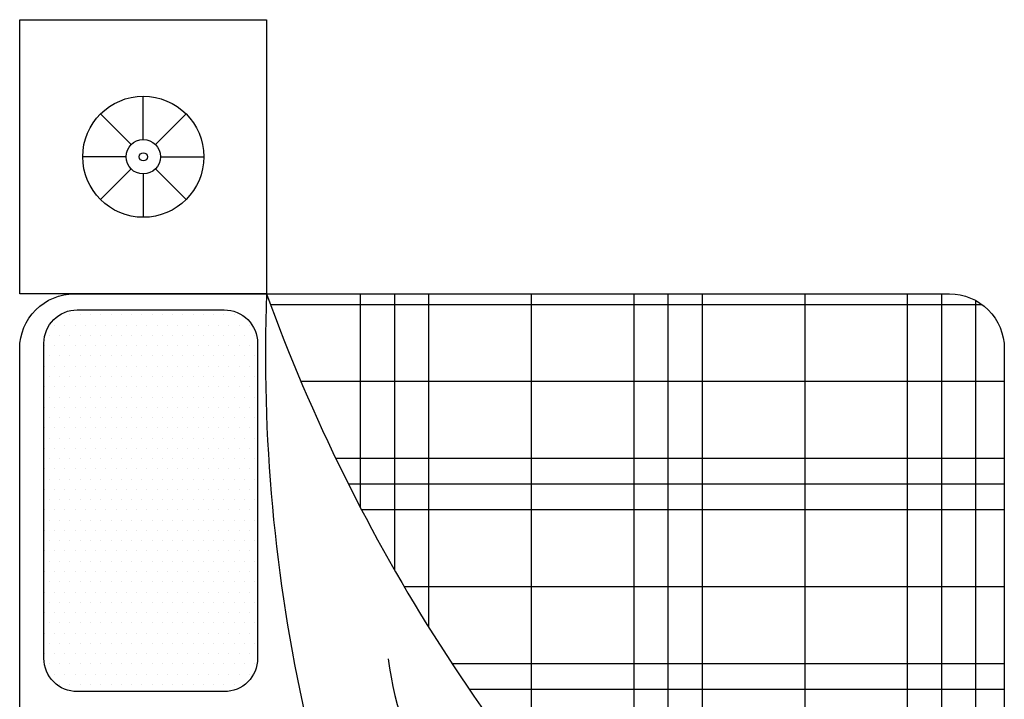
# Model space of a CAD drawing. Units: inches. Extents: x 528 to 2520, y -151 to 1354.
# Tile 19 of 41: x 1137 to 1192, y 1189 to 1227. Entities that reach past the tile are written whole.
import ezdxf

# ---------------------------------------------------------------- set-up
doc = ezdxf.new("R2010")
doc.units = ezdxf.units.IN
doc.header["$MEASUREMENT"] = 0
doc.layers.add('A-FURN', color=8, linetype='Continuous', lineweight=18)
doc.layers.add('BLOCK', color=6, linetype='Continuous')

# ---------------------------------------------------------------- blocks, each defined once
blk = doc.blocks.new('*X15')
at = {"color": 0}
for p, q in [((276.598, 451.25), (280.51, 451.25)), ((275.455, 450.625), (280.51, 450.625)), ((274.411, 450), (280.51, 450)), ((265.51, 448.125), (267.634, 448.125)), ((271.723, 448.125), (280.51, 448.125)), ((265.51, 446.25), (268.465, 446.25)), ((269.519, 446.25), (280.51, 446.25)), ((265.51, 445.625), (268.531, 445.625)), ((268.866, 445.625), (280.51, 445.625)), ((265.51, 445), (280.51, 445)), ((265.51, 443.125), (280.51, 443.125)), ((265.51, 441.25), (280.51, 441.25)), ((265.51, 440.625), (280.51, 440.625)), ((265.634, 440), (280.386, 440))]:
    blk.add_line(p, q, dxfattribs=at)
blk = doc.blocks.new('*X16')
at = {"color": 0}
for p, q in [((280.312, 439.886), (280.312, 452.896)), ((278.906, 439.482), (278.906, 452.338)), ((277.5, 439.482), (277.5, 451.702)), ((277.031, 439.482), (277.031, 451.471)), ((276.562, 439.482), (276.562, 451.231)), ((275.156, 439.482), (275.156, 450.451)), ((265.781, 439.797), (265.781, 449.511)), ((273.75, 439.482), (273.75, 449.576)), ((266.25, 439.517), (266.25, 449.296)), ((273.281, 439.482), (273.281, 449.261)), ((272.812, 439.482), (272.812, 448.934)), ((267.656, 439.482), (267.656, 448.095)), ((271.406, 439.482), (271.406, 447.876)), ((270, 439.482), (270, 446.689)), ((269.531, 439.482), (269.531, 446.262)), ((269.062, 439.482), (269.062, 445.817))]:
    blk.add_line(p, q, dxfattribs=at)
blk = doc.blocks.new('*X17')
at = {"color": 0}
for p, q in [((273.9375, 457.03125), (273.9375, 457.03125)), ((274.3125, 457.03125), (274.3125, 457.03125)), ((274.6875, 457.03125), (274.6875, 457.03125)), ((275.0625, 457.03125), (275.0625, 457.03125)), ((275.4375, 457.03125), (275.4375, 457.03125)), ((275.8125, 457.03125), (275.8125, 457.03125)), ((276.1875, 457.03125), (276.1875, 457.03125)), ((276.5625, 457.03125), (276.5625, 457.03125)), ((276.9375, 457.03125), (276.9375, 457.03125)), ((277.3125, 457.03125), (277.3125, 457.03125)), ((277.6875, 457.03125), (277.6875, 457.03125)), ((278.0625, 457.03125), (278.0625, 457.03125)), ((278.4375, 457.03125), (278.4375, 457.03125)), ((278.8125, 457.03125), (278.8125, 457.03125)), ((279.1875, 457.03125), (279.1875, 457.03125)), ((279.5625, 457.03125), (279.5625, 457.03125)), ((273.5625, 456.84375), (273.5625, 456.84375)), ((273.75, 456.9375), (273.75, 456.9375)), ((273.9375, 456.84375), (273.9375, 456.84375)), ((274.125, 456.9375), (274.125, 456.9375)), ((274.3125, 456.84375), (274.3125, 456.84375)), ((274.5, 456.9375), (274.5, 456.9375)), ((274.6875, 456.84375), (274.6875, 456.84375)), ((274.875, 456.9375), (274.875, 456.9375)), ((275.0625, 456.84375), (275.0625, 456.84375)), ((275.25, 456.9375), (275.25, 456.9375)), ((275.4375, 456.84375), (275.4375, 456.84375)), ((275.625, 456.9375), (275.625, 456.9375)), ((275.8125, 456.84375), (275.8125, 456.84375)), ((276, 456.9375), (276, 456.9375)), ((276.1875, 456.84375), (276.1875, 456.84375)), ((276.375, 456.9375), (276.375, 456.9375)), ((276.5625, 456.84375), (276.5625, 456.84375)), ((276.75, 456.9375), (276.75, 456.9375)), ((276.9375, 456.84375), (276.9375, 456.84375)), ((277.125, 456.9375), (277.125, 456.9375)), ((277.3125, 456.84375), (277.3125, 456.84375)), ((277.5, 456.9375), (277.5, 456.9375)), ((277.6875, 456.84375), (277.6875, 456.84375)), ((277.875, 456.9375), (277.875, 456.9375)), ((278.0625, 456.84375), (278.0625, 456.84375)), ((278.25, 456.9375), (278.25, 456.9375)), ((278.4375, 456.84375), (278.4375, 456.84375)), ((278.625, 456.9375), (278.625, 456.9375)), ((278.8125, 456.84375), (278.8125, 456.84375)), ((279, 456.9375), (279, 456.9375)), ((279.1875, 456.84375), (279.1875, 456.84375)), ((279.375, 456.9375), (279.375, 456.9375)), ((279.5625, 456.84375), (279.5625, 456.84375)), ((279.75, 456.9375), (279.75, 456.9375)), ((279.9375, 456.84375), (279.9375, 456.84375)), ((273.375, 456.75), (273.375, 456.75)), ((273.75, 456.75), (273.75, 456.75)), ((274.125, 456.75), (274.125, 456.75)), ((274.5, 456.75), (274.5, 456.75)), ((274.875, 456.75), (274.875, 456.75)), ((275.25, 456.75), (275.25, 456.75)), ((275.625, 456.75), (275.625, 456.75)), ((276, 456.75), (276, 456.75)), ((276.375, 456.75), (276.375, 456.75)), ((276.75, 456.75), (276.75, 456.75)), ((277.125, 456.75), (277.125, 456.75)), ((277.5, 456.75), (277.5, 456.75)), ((277.875, 456.75), (277.875, 456.75)), ((278.25, 456.75), (278.25, 456.75)), ((278.625, 456.75), (278.625, 456.75)), ((279, 456.75), (279, 456.75)), ((279.375, 456.75), (279.375, 456.75)), ((279.75, 456.75), (279.75, 456.75)), ((280.125, 456.75), (280.125, 456.75)), ((273.375, 456.5625), (273.375, 456.5625)), ((273.5625, 456.65625), (273.5625, 456.65625)), ((273.75, 456.5625), (273.75, 456.5625)), ((273.9375, 456.65625), (273.9375, 456.65625)), ((274.125, 456.5625), (274.125, 456.5625)), ((274.3125, 456.65625), (274.3125, 456.65625)), ((274.5, 456.5625), (274.5, 456.5625)), ((274.6875, 456.65625), (274.6875, 456.65625)), ((274.875, 456.5625), (274.875, 456.5625)), ((275.0625, 456.65625), (275.0625, 456.65625)), ((275.25, 456.5625), (275.25, 456.5625)), ((275.4375, 456.65625), (275.4375, 456.65625)), ((275.625, 456.5625), (275.625, 456.5625)), ((275.8125, 456.65625), (275.8125, 456.65625)), ((276, 456.5625), (276, 456.5625)), ((276.1875, 456.65625), (276.1875, 456.65625)), ((276.375, 456.5625), (276.375, 456.5625)), ((276.5625, 456.65625), (276.5625, 456.65625)), ((276.75, 456.5625), (276.75, 456.5625)), ((276.9375, 456.65625), (276.9375, 456.65625)), ((277.125, 456.5625), (277.125, 456.5625)), ((277.3125, 456.65625), (277.3125, 456.65625)), ((277.5, 456.5625), (277.5, 456.5625)), ((277.6875, 456.65625), (277.6875, 456.65625)), ((277.875, 456.5625), (277.875, 456.5625)), ((278.0625, 456.65625), (278.0625, 456.65625)), ((278.25, 456.5625), (278.25, 456.5625)), ((278.4375, 456.65625), (278.4375, 456.65625)), ((278.625, 456.5625), (278.625, 456.5625)), ((278.8125, 456.65625), (278.8125, 456.65625)), ((279, 456.5625), (279, 456.5625)), ((279.1875, 456.65625), (279.1875, 456.65625)), ((279.375, 456.5625), (279.375, 456.5625)), ((279.5625, 456.65625), (279.5625, 456.65625)), ((279.75, 456.5625), (279.75, 456.5625)), ((279.9375, 456.65625), (279.9375, 456.65625)), ((280.125, 456.5625), (280.125, 456.5625)), ((273.375, 456.375), (273.375, 456.375)), ((273.5625, 456.46875), (273.5625, 456.46875)), ((273.75, 456.375), (273.75, 456.375)), ((273.9375, 456.46875), (273.9375, 456.46875)), ((274.125, 456.375), (274.125, 456.375)), ((274.3125, 456.46875), (274.3125, 456.46875)), ((274.5, 456.375), (274.5, 456.375)), ((274.6875, 456.46875), (274.6875, 456.46875)), ((274.875, 456.375), (274.875, 456.375)), ((275.0625, 456.46875), (275.0625, 456.46875)), ((275.25, 456.375), (275.25, 456.375)), ((275.4375, 456.46875), (275.4375, 456.46875)), ((275.625, 456.375), (275.625, 456.375)), ((275.8125, 456.46875), (275.8125, 456.46875)), ((276, 456.375), (276, 456.375)), ((276.1875, 456.46875), (276.1875, 456.46875)), ((276.375, 456.375), (276.375, 456.375)), ((276.5625, 456.46875), (276.5625, 456.46875)), ((276.75, 456.375), (276.75, 456.375)), ((276.9375, 456.46875), (276.9375, 456.46875)), ((277.125, 456.375), (277.125, 456.375)), ((277.3125, 456.46875), (277.3125, 456.46875)), ((277.5, 456.375), (277.5, 456.375)), ((277.6875, 456.46875), (277.6875, 456.46875)), ((277.875, 456.375), (277.875, 456.375)), ((278.0625, 456.46875), (278.0625, 456.46875)), ((278.25, 456.375), (278.25, 456.375)), ((278.4375, 456.46875), (278.4375, 456.46875)), ((278.625, 456.375), (278.625, 456.375)), ((278.8125, 456.46875), (278.8125, 456.46875)), ((279, 456.375), (279, 456.375)), ((279.1875, 456.46875), (279.1875, 456.46875)), ((279.375, 456.375), (279.375, 456.375)), ((279.5625, 456.46875), (279.5625, 456.46875)), ((279.75, 456.375), (279.75, 456.375)), ((279.9375, 456.46875), (279.9375, 456.46875)), ((280.125, 456.375), (280.125, 456.375)), ((273.375, 456.1875), (273.375, 456.1875)), ((273.5625, 456.28125), (273.5625, 456.28125)), ((273.75, 456.1875), (273.75, 456.1875)), ((273.9375, 456.28125), (273.9375, 456.28125)), ((274.125, 456.1875), (274.125, 456.1875)), ((274.3125, 456.28125), (274.3125, 456.28125)), ((274.5, 456.1875), (274.5, 456.1875)), ((274.6875, 456.28125), (274.6875, 456.28125)), ((274.875, 456.1875), (274.875, 456.1875)), ((275.0625, 456.28125), (275.0625, 456.28125)), ((275.25, 456.1875), (275.25, 456.1875)), ((275.4375, 456.28125), (275.4375, 456.28125)), ((275.625, 456.1875), (275.625, 456.1875)), ((275.8125, 456.28125), (275.8125, 456.28125)), ((276, 456.1875), (276, 456.1875)), ((276.1875, 456.28125), (276.1875, 456.28125)), ((276.375, 456.1875), (276.375, 456.1875)), ((276.5625, 456.28125), (276.5625, 456.28125)), ((276.75, 456.1875), (276.75, 456.1875)), ((276.9375, 456.28125), (276.9375, 456.28125)), ((277.125, 456.1875), (277.125, 456.1875)), ((277.3125, 456.28125), (277.3125, 456.28125)), ((277.5, 456.1875), (277.5, 456.1875)), ((277.6875, 456.28125), (277.6875, 456.28125)), ((277.875, 456.1875), (277.875, 456.1875)), ((278.0625, 456.28125), (278.0625, 456.28125)), ((278.25, 456.1875), (278.25, 456.1875)), ((278.4375, 456.28125), (278.4375, 456.28125)), ((278.625, 456.1875), (278.625, 456.1875)), ((278.8125, 456.28125), (278.8125, 456.28125)), ((279, 456.1875), (279, 456.1875)), ((279.1875, 456.28125), (279.1875, 456.28125)), ((279.375, 456.1875), (279.375, 456.1875)), ((279.5625, 456.28125), (279.5625, 456.28125)), ((279.75, 456.1875), (279.75, 456.1875)), ((279.9375, 456.28125), (279.9375, 456.28125)), ((280.125, 456.1875), (280.125, 456.1875)), ((273.375, 456), (273.375, 456)), ((273.5625, 456.09375), (273.5625, 456.09375)), ((273.75, 456), (273.75, 456)), ((273.9375, 456.09375), (273.9375, 456.09375)), ((274.125, 456), (274.125, 456)), ((274.3125, 456.09375), (274.3125, 456.09375)), ((274.5, 456), (274.5, 456)), ((274.6875, 456.09375), (274.6875, 456.09375)), ((274.875, 456), (274.875, 456)), ((275.0625, 456.09375), (275.0625, 456.09375)), ((275.25, 456), (275.25, 456)), ((275.4375, 456.09375), (275.4375, 456.09375)), ((275.625, 456), (275.625, 456)), ((275.8125, 456.09375), (275.8125, 456.09375)), ((276, 456), (276, 456)), ((276.1875, 456.09375), (276.1875, 456.09375)), ((276.375, 456), (276.375, 456)), ((276.5625, 456.09375), (276.5625, 456.09375)), ((276.75, 456), (276.75, 456)), ((276.9375, 456.09375), (276.9375, 456.09375)), ((277.125, 456), (277.125, 456)), ((277.3125, 456.09375), (277.3125, 456.09375)), ((277.5, 456), (277.5, 456)), ((277.6875, 456.09375), (277.6875, 456.09375)), ((277.875, 456), (277.875, 456)), ((278.0625, 456.09375), (278.0625, 456.09375)), ((278.25, 456), (278.25, 456)), ((278.4375, 456.09375), (278.4375, 456.09375)), ((278.625, 456), (278.625, 456)), ((278.8125, 456.09375), (278.8125, 456.09375)), ((279, 456), (279, 456)), ((279.1875, 456.09375), (279.1875, 456.09375)), ((279.375, 456), (279.375, 456)), ((279.5625, 456.09375), (279.5625, 456.09375)), ((279.75, 456), (279.75, 456)), ((279.9375, 456.09375), (279.9375, 456.09375)), ((280.125, 456), (280.125, 456)), ((273.375, 455.8125), (273.375, 455.8125)), ((273.5625, 455.90625), (273.5625, 455.90625)), ((273.75, 455.8125), (273.75, 455.8125)), ((273.9375, 455.90625), (273.9375, 455.90625)), ((274.125, 455.8125), (274.125, 455.8125)), ((274.3125, 455.90625), (274.3125, 455.90625)), ((274.5, 455.8125), (274.5, 455.8125)), ((274.6875, 455.90625), (274.6875, 455.90625)), ((274.875, 455.8125), (274.875, 455.8125)), ((275.0625, 455.90625), (275.0625, 455.90625)), ((275.25, 455.8125), (275.25, 455.8125)), ((275.4375, 455.90625), (275.4375, 455.90625)), ((275.625, 455.8125), (275.625, 455.8125)), ((275.8125, 455.90625), (275.8125, 455.90625)), ((276, 455.8125), (276, 455.8125)), ((276.1875, 455.90625), (276.1875, 455.90625)), ((276.375, 455.8125), (276.375, 455.8125)), ((276.5625, 455.90625), (276.5625, 455.90625)), ((276.75, 455.8125), (276.75, 455.8125)), ((276.9375, 455.90625), (276.9375, 455.90625)), ((277.125, 455.8125), (277.125, 455.8125)), ((277.3125, 455.90625), (277.3125, 455.90625)), ((277.5, 455.8125), (277.5, 455.8125)), ((277.6875, 455.90625), (277.6875, 455.90625)), ((277.875, 455.8125), (277.875, 455.8125)), ((278.0625, 455.90625), (278.0625, 455.90625)), ((278.25, 455.8125), (278.25, 455.8125)), ((278.4375, 455.90625), (278.4375, 455.90625)), ((278.625, 455.8125), (278.625, 455.8125)), ((278.8125, 455.90625), (278.8125, 455.90625)), ((279, 455.8125), (279, 455.8125)), ((279.1875, 455.90625), (279.1875, 455.90625)), ((279.375, 455.8125), (279.375, 455.8125)), ((279.5625, 455.90625), (279.5625, 455.90625)), ((279.75, 455.8125), (279.75, 455.8125)), ((279.9375, 455.90625), (279.9375, 455.90625)), ((280.125, 455.8125), (280.125, 455.8125)), ((273.375, 455.625), (273.375, 455.625)), ((273.5625, 455.71875), (273.5625, 455.71875)), ((273.75, 455.625), (273.75, 455.625)), ((273.9375, 455.71875), (273.9375, 455.71875)), ((274.125, 455.625), (274.125, 455.625)), ((274.3125, 455.71875), (274.3125, 455.71875)), ((274.5, 455.625), (274.5, 455.625)), ((274.6875, 455.71875), (274.6875, 455.71875)), ((274.875, 455.625), (274.875, 455.625)), ((275.0625, 455.71875), (275.0625, 455.71875)), ((275.25, 455.625), (275.25, 455.625)), ((275.4375, 455.71875), (275.4375, 455.71875)), ((275.625, 455.625), (275.625, 455.625)), ((275.8125, 455.71875), (275.8125, 455.71875)), ((276, 455.625), (276, 455.625)), ((276.1875, 455.71875), (276.1875, 455.71875)), ((276.375, 455.625), (276.375, 455.625)), ((276.5625, 455.71875), (276.5625, 455.71875)), ((276.75, 455.625), (276.75, 455.625)), ((276.9375, 455.71875), (276.9375, 455.71875)), ((277.125, 455.625), (277.125, 455.625)), ((277.3125, 455.71875), (277.3125, 455.71875)), ((277.5, 455.625), (277.5, 455.625)), ((277.6875, 455.71875), (277.6875, 455.71875)), ((277.875, 455.625), (277.875, 455.625)), ((278.0625, 455.71875), (278.0625, 455.71875)), ((278.25, 455.625), (278.25, 455.625)), ((278.4375, 455.71875), (278.4375, 455.71875)), ((278.625, 455.625), (278.625, 455.625)), ((278.8125, 455.71875), (278.8125, 455.71875)), ((279, 455.625), (279, 455.625)), ((279.1875, 455.71875), (279.1875, 455.71875)), ((279.375, 455.625), (279.375, 455.625)), ((279.5625, 455.71875), (279.5625, 455.71875)), ((279.75, 455.625), (279.75, 455.625)), ((279.9375, 455.71875), (279.9375, 455.71875)), ((280.125, 455.625), (280.125, 455.625)), ((273.375, 455.4375), (273.375, 455.4375)), ((273.5625, 455.53125), (273.5625, 455.53125)), ((273.75, 455.4375), (273.75, 455.4375)), ((273.9375, 455.53125), (273.9375, 455.53125)), ((274.125, 455.4375), (274.125, 455.4375)), ((274.3125, 455.53125), (274.3125, 455.53125)), ((274.5, 455.4375), (274.5, 455.4375)), ((274.6875, 455.53125), (274.6875, 455.53125)), ((274.875, 455.4375), (274.875, 455.4375)), ((275.0625, 455.53125), (275.0625, 455.53125)), ((275.25, 455.4375), (275.25, 455.4375)), ((275.4375, 455.53125), (275.4375, 455.53125)), ((275.625, 455.4375), (275.625, 455.4375)), ((275.8125, 455.53125), (275.8125, 455.53125)), ((276, 455.4375), (276, 455.4375)), ((276.1875, 455.53125), (276.1875, 455.53125)), ((276.375, 455.4375), (276.375, 455.4375)), ((276.5625, 455.53125), (276.5625, 455.53125)), ((276.75, 455.4375), (276.75, 455.4375)), ((276.9375, 455.53125), (276.9375, 455.53125)), ((277.125, 455.4375), (277.125, 455.4375)), ((277.3125, 455.53125), (277.3125, 455.53125)), ((277.5, 455.4375), (277.5, 455.4375)), ((277.6875, 455.53125), (277.6875, 455.53125)), ((277.875, 455.4375), (277.875, 455.4375)), ((278.0625, 455.53125), (278.0625, 455.53125)), ((278.25, 455.4375), (278.25, 455.4375)), ((278.4375, 455.53125), (278.4375, 455.53125)), ((278.625, 455.4375), (278.625, 455.4375)), ((278.8125, 455.53125), (278.8125, 455.53125)), ((279, 455.4375), (279, 455.4375)), ((279.1875, 455.53125), (279.1875, 455.53125)), ((279.375, 455.4375), (279.375, 455.4375)), ((279.5625, 455.53125), (279.5625, 455.53125)), ((279.75, 455.4375), (279.75, 455.4375)), ((279.9375, 455.53125), (279.9375, 455.53125)), ((280.125, 455.4375), (280.125, 455.4375)), ((273.375, 455.25), (273.375, 455.25)), ((273.5625, 455.34375), (273.5625, 455.34375)), ((273.75, 455.25), (273.75, 455.25)), ((273.9375, 455.34375), (273.9375, 455.34375)), ((274.125, 455.25), (274.125, 455.25)), ((274.3125, 455.34375), (274.3125, 455.34375)), ((274.5, 455.25), (274.5, 455.25)), ((274.6875, 455.34375), (274.6875, 455.34375)), ((274.875, 455.25), (274.875, 455.25)), ((275.0625, 455.34375), (275.0625, 455.34375)), ((275.25, 455.25), (275.25, 455.25)), ((275.4375, 455.34375), (275.4375, 455.34375)), ((275.625, 455.25), (275.625, 455.25)), ((275.8125, 455.34375), (275.8125, 455.34375)), ((276, 455.25), (276, 455.25)), ((276.1875, 455.34375), (276.1875, 455.34375)), ((276.375, 455.25), (276.375, 455.25)), ((276.5625, 455.34375), (276.5625, 455.34375)), ((276.75, 455.25), (276.75, 455.25)), ((276.9375, 455.34375), (276.9375, 455.34375)), ((277.125, 455.25), (277.125, 455.25)), ((277.3125, 455.34375), (277.3125, 455.34375)), ((277.5, 455.25), (277.5, 455.25)), ((277.6875, 455.34375), (277.6875, 455.34375)), ((277.875, 455.25), (277.875, 455.25)), ((278.0625, 455.34375), (278.0625, 455.34375)), ((278.25, 455.25), (278.25, 455.25)), ((278.4375, 455.34375), (278.4375, 455.34375)), ((278.625, 455.25), (278.625, 455.25)), ((278.8125, 455.34375), (278.8125, 455.34375)), ((279, 455.25), (279, 455.25)), ((279.1875, 455.34375), (279.1875, 455.34375)), ((279.375, 455.25), (279.375, 455.25)), ((279.5625, 455.34375), (279.5625, 455.34375)), ((279.75, 455.25), (279.75, 455.25)), ((279.9375, 455.34375), (279.9375, 455.34375)), ((280.125, 455.25), (280.125, 455.25)), ((273.375, 455.0625), (273.375, 455.0625)), ((273.5625, 455.15625), (273.5625, 455.15625)), ((273.75, 455.0625), (273.75, 455.0625)), ((273.9375, 455.15625), (273.9375, 455.15625)), ((274.125, 455.0625), (274.125, 455.0625)), ((274.3125, 455.15625), (274.3125, 455.15625)), ((274.5, 455.0625), (274.5, 455.0625)), ((274.6875, 455.15625), (274.6875, 455.15625)), ((274.875, 455.0625), (274.875, 455.0625)), ((275.0625, 455.15625), (275.0625, 455.15625)), ((275.25, 455.0625), (275.25, 455.0625)), ((275.4375, 455.15625), (275.4375, 455.15625)), ((275.625, 455.0625), (275.625, 455.0625)), ((275.8125, 455.15625), (275.8125, 455.15625)), ((276, 455.0625), (276, 455.0625)), ((276.1875, 455.15625), (276.1875, 455.15625)), ((276.375, 455.0625), (276.375, 455.0625)), ((276.5625, 455.15625), (276.5625, 455.15625)), ((276.75, 455.0625), (276.75, 455.0625)), ((276.9375, 455.15625), (276.9375, 455.15625)), ((277.125, 455.0625), (277.125, 455.0625)), ((277.3125, 455.15625), (277.3125, 455.15625)), ((277.5, 455.0625), (277.5, 455.0625)), ((277.6875, 455.15625), (277.6875, 455.15625)), ((277.875, 455.0625), (277.875, 455.0625)), ((278.0625, 455.15625), (278.0625, 455.15625)), ((278.25, 455.0625), (278.25, 455.0625)), ((278.4375, 455.15625), (278.4375, 455.15625)), ((278.625, 455.0625), (278.625, 455.0625)), ((278.8125, 455.15625), (278.8125, 455.15625)), ((279, 455.0625), (279, 455.0625)), ((279.1875, 455.15625), (279.1875, 455.15625)), ((279.375, 455.0625), (279.375, 455.0625)), ((279.5625, 455.15625), (279.5625, 455.15625)), ((279.75, 455.0625), (279.75, 455.0625)), ((279.9375, 455.15625), (279.9375, 455.15625)), ((280.125, 455.0625), (280.125, 455.0625)), ((273.375, 454.875), (273.375, 454.875)), ((273.5625, 454.96875), (273.5625, 454.96875)), ((273.75, 454.875), (273.75, 454.875)), ((273.9375, 454.96875), (273.9375, 454.96875)), ((274.125, 454.875), (274.125, 454.875)), ((274.3125, 454.96875), (274.3125, 454.96875)), ((274.5, 454.875), (274.5, 454.875)), ((274.6875, 454.96875), (274.6875, 454.96875)), ((274.875, 454.875), (274.875, 454.875)), ((275.0625, 454.96875), (275.0625, 454.96875)), ((275.25, 454.875), (275.25, 454.875)), ((275.4375, 454.96875), (275.4375, 454.96875)), ((275.625, 454.875), (275.625, 454.875)), ((275.8125, 454.96875), (275.8125, 454.96875)), ((276, 454.875), (276, 454.875)), ((276.1875, 454.96875), (276.1875, 454.96875)), ((276.375, 454.875), (276.375, 454.875)), ((276.5625, 454.96875), (276.5625, 454.96875)), ((276.75, 454.875), (276.75, 454.875)), ((276.9375, 454.96875), (276.9375, 454.96875)), ((277.125, 454.875), (277.125, 454.875)), ((277.3125, 454.96875), (277.3125, 454.96875)), ((277.5, 454.875), (277.5, 454.875)), ((277.6875, 454.96875), (277.6875, 454.96875)), ((277.875, 454.875), (277.875, 454.875)), ((278.0625, 454.96875), (278.0625, 454.96875)), ((278.25, 454.875), (278.25, 454.875)), ((278.4375, 454.96875), (278.4375, 454.96875)), ((278.625, 454.875), (278.625, 454.875)), ((278.8125, 454.96875), (278.8125, 454.96875)), ((279, 454.875), (279, 454.875)), ((279.1875, 454.96875), (279.1875, 454.96875)), ((279.375, 454.875), (279.375, 454.875)), ((279.5625, 454.96875), (279.5625, 454.96875)), ((279.75, 454.875), (279.75, 454.875)), ((279.9375, 454.96875), (279.9375, 454.96875)), ((280.125, 454.875), (280.125, 454.875)), ((273.375, 454.6875), (273.375, 454.6875)), ((273.5625, 454.78125), (273.5625, 454.78125)), ((273.75, 454.6875), (273.75, 454.6875)), ((273.9375, 454.78125), (273.9375, 454.78125)), ((274.125, 454.6875), (274.125, 454.6875)), ((274.3125, 454.78125), (274.3125, 454.78125)), ((274.5, 454.6875), (274.5, 454.6875)), ((274.6875, 454.78125), (274.6875, 454.78125)), ((274.875, 454.6875), (274.875, 454.6875)), ((275.0625, 454.78125), (275.0625, 454.78125)), ((275.25, 454.6875), (275.25, 454.6875)), ((275.4375, 454.78125), (275.4375, 454.78125)), ((275.625, 454.6875), (275.625, 454.6875)), ((275.8125, 454.78125), (275.8125, 454.78125)), ((276, 454.6875), (276, 454.6875)), ((276.1875, 454.78125), (276.1875, 454.78125)), ((276.375, 454.6875), (276.375, 454.6875)), ((276.5625, 454.78125), (276.5625, 454.78125)), ((276.75, 454.6875), (276.75, 454.6875)), ((276.9375, 454.78125), (276.9375, 454.78125)), ((277.125, 454.6875), (277.125, 454.6875)), ((277.3125, 454.78125), (277.3125, 454.78125)), ((277.5, 454.6875), (277.5, 454.6875)), ((277.6875, 454.78125), (277.6875, 454.78125)), ((277.875, 454.6875), (277.875, 454.6875)), ((278.0625, 454.78125), (278.0625, 454.78125)), ((278.25, 454.6875), (278.25, 454.6875)), ((278.4375, 454.78125), (278.4375, 454.78125)), ((278.625, 454.6875), (278.625, 454.6875)), ((278.8125, 454.78125), (278.8125, 454.78125)), ((279, 454.6875), (279, 454.6875)), ((279.1875, 454.78125), (279.1875, 454.78125)), ((279.375, 454.6875), (279.375, 454.6875)), ((279.5625, 454.78125), (279.5625, 454.78125)), ((279.75, 454.6875), (279.75, 454.6875)), ((279.9375, 454.78125), (279.9375, 454.78125)), ((280.125, 454.6875), (280.125, 454.6875)), ((273.5625, 454.59375), (273.5625, 454.59375)), ((273.9375, 454.59375), (273.9375, 454.59375)), ((274.3125, 454.59375), (274.3125, 454.59375)), ((274.6875, 454.59375), (274.6875, 454.59375)), ((275.0625, 454.59375), (275.0625, 454.59375)), ((275.4375, 454.59375), (275.4375, 454.59375)), ((275.8125, 454.59375), (275.8125, 454.59375)), ((276.1875, 454.59375), (276.1875, 454.59375)), ((276.5625, 454.59375), (276.5625, 454.59375)), ((276.9375, 454.59375), (276.9375, 454.59375)), ((277.3125, 454.59375), (277.3125, 454.59375)), ((277.6875, 454.59375), (277.6875, 454.59375)), ((278.0625, 454.59375), (278.0625, 454.59375)), ((278.4375, 454.59375), (278.4375, 454.59375)), ((278.8125, 454.59375), (278.8125, 454.59375)), ((279.1875, 454.59375), (279.1875, 454.59375)), ((279.5625, 454.59375), (279.5625, 454.59375)), ((279.9375, 454.59375), (279.9375, 454.59375)), ((273.375, 454.5), (273.375, 454.5)), ((273.5625, 454.40625), (273.5625, 454.40625)), ((273.75, 454.5), (273.75, 454.5)), ((273.9375, 454.40625), (273.9375, 454.40625)), ((274.125, 454.5), (274.125, 454.5)), ((274.3125, 454.40625), (274.3125, 454.40625)), ((274.5, 454.5), (274.5, 454.5)), ((274.6875, 454.40625), (274.6875, 454.40625)), ((274.875, 454.5), (274.875, 454.5)), ((275.0625, 454.40625), (275.0625, 454.40625)), ((275.25, 454.5), (275.25, 454.5)), ((275.4375, 454.40625), (275.4375, 454.40625)), ((275.625, 454.5), (275.625, 454.5)), ((275.8125, 454.40625), (275.8125, 454.40625)), ((276, 454.5), (276, 454.5)), ((276.1875, 454.40625), (276.1875, 454.40625)), ((276.375, 454.5), (276.375, 454.5)), ((276.5625, 454.40625), (276.5625, 454.40625)), ((276.75, 454.5), (276.75, 454.5)), ((276.9375, 454.40625), (276.9375, 454.40625)), ((277.125, 454.5), (277.125, 454.5)), ((277.3125, 454.40625), (277.3125, 454.40625)), ((277.5, 454.5), (277.5, 454.5)), ((277.6875, 454.40625), (277.6875, 454.40625)), ((277.875, 454.5), (277.875, 454.5)), ((278.0625, 454.40625), (278.0625, 454.40625)), ((278.25, 454.5), (278.25, 454.5)), ((278.4375, 454.40625), (278.4375, 454.40625)), ((278.625, 454.5), (278.625, 454.5)), ((278.8125, 454.40625), (278.8125, 454.40625)), ((279, 454.5), (279, 454.5)), ((279.1875, 454.40625), (279.1875, 454.40625)), ((279.375, 454.5), (279.375, 454.5)), ((279.5625, 454.40625), (279.5625, 454.40625)), ((279.75, 454.5), (279.75, 454.5)), ((279.9375, 454.40625), (279.9375, 454.40625)), ((280.125, 454.5), (280.125, 454.5)), ((273.375, 454.3125), (273.375, 454.3125)), ((273.5625, 454.21875), (273.5625, 454.21875)), ((273.75, 454.3125), (273.75, 454.3125)), ((273.9375, 454.21875), (273.9375, 454.21875)), ((274.125, 454.3125), (274.125, 454.3125)), ((274.3125, 454.21875), (274.3125, 454.21875)), ((274.5, 454.3125), (274.5, 454.3125)), ((274.6875, 454.21875), (274.6875, 454.21875)), ((274.875, 454.3125), (274.875, 454.3125)), ((275.0625, 454.21875), (275.0625, 454.21875)), ((275.25, 454.3125), (275.25, 454.3125)), ((275.4375, 454.21875), (275.4375, 454.21875)), ((275.625, 454.3125), (275.625, 454.3125)), ((275.8125, 454.21875), (275.8125, 454.21875)), ((276, 454.3125), (276, 454.3125)), ((276.1875, 454.21875), (276.1875, 454.21875)), ((276.375, 454.3125), (276.375, 454.3125)), ((276.5625, 454.21875), (276.5625, 454.21875)), ((276.75, 454.3125), (276.75, 454.3125)), ((276.9375, 454.21875), (276.9375, 454.21875)), ((277.125, 454.3125), (277.125, 454.3125)), ((277.3125, 454.21875), (277.3125, 454.21875)), ((277.5, 454.3125), (277.5, 454.3125)), ((277.6875, 454.21875), (277.6875, 454.21875)), ((277.875, 454.3125), (277.875, 454.3125)), ((278.0625, 454.21875), (278.0625, 454.21875)), ((278.25, 454.3125), (278.25, 454.3125)), ((278.4375, 454.21875), (278.4375, 454.21875)), ((278.625, 454.3125), (278.625, 454.3125)), ((278.8125, 454.21875), (278.8125, 454.21875)), ((279, 454.3125), (279, 454.3125)), ((279.1875, 454.21875), (279.1875, 454.21875)), ((279.375, 454.3125), (279.375, 454.3125)), ((279.5625, 454.21875), (279.5625, 454.21875)), ((279.75, 454.3125), (279.75, 454.3125)), ((279.9375, 454.21875), (279.9375, 454.21875)), ((280.125, 454.3125), (280.125, 454.3125)), ((273.375, 454.125), (273.375, 454.125)), ((273.5625, 454.03125), (273.5625, 454.03125)), ((273.75, 454.125), (273.75, 454.125)), ((273.9375, 454.03125), (273.9375, 454.03125)), ((274.125, 454.125), (274.125, 454.125)), ((274.3125, 454.03125), (274.3125, 454.03125)), ((274.5, 454.125), (274.5, 454.125)), ((274.6875, 454.03125), (274.6875, 454.03125)), ((274.875, 454.125), (274.875, 454.125)), ((275.0625, 454.03125), (275.0625, 454.03125)), ((275.25, 454.125), (275.25, 454.125)), ((275.4375, 454.03125), (275.4375, 454.03125)), ((275.625, 454.125), (275.625, 454.125)), ((275.8125, 454.03125), (275.8125, 454.03125)), ((276, 454.125), (276, 454.125)), ((276.1875, 454.03125), (276.1875, 454.03125)), ((276.375, 454.125), (276.375, 454.125)), ((276.5625, 454.03125), (276.5625, 454.03125)), ((276.75, 454.125), (276.75, 454.125)), ((276.9375, 454.03125), (276.9375, 454.03125)), ((277.125, 454.125), (277.125, 454.125)), ((277.3125, 454.03125), (277.3125, 454.03125)), ((277.5, 454.125), (277.5, 454.125)), ((277.6875, 454.03125), (277.6875, 454.03125)), ((277.875, 454.125), (277.875, 454.125)), ((278.0625, 454.03125), (278.0625, 454.03125)), ((278.25, 454.125), (278.25, 454.125)), ((278.4375, 454.03125), (278.4375, 454.03125)), ((278.625, 454.125), (278.625, 454.125)), ((278.8125, 454.03125), (278.8125, 454.03125)), ((279, 454.125), (279, 454.125)), ((279.1875, 454.03125), (279.1875, 454.03125)), ((279.375, 454.125), (279.375, 454.125)), ((279.5625, 454.03125), (279.5625, 454.03125)), ((279.75, 454.125), (279.75, 454.125)), ((279.9375, 454.03125), (279.9375, 454.03125)), ((280.125, 454.125), (280.125, 454.125)), ((273.375, 453.9375), (273.375, 453.9375)), ((273.5625, 453.84375), (273.5625, 453.84375)), ((273.75, 453.9375), (273.75, 453.9375)), ((273.9375, 453.84375), (273.9375, 453.84375)), ((274.125, 453.9375), (274.125, 453.9375)), ((274.3125, 453.84375), (274.3125, 453.84375)), ((274.5, 453.9375), (274.5, 453.9375)), ((274.6875, 453.84375), (274.6875, 453.84375)), ((274.875, 453.9375), (274.875, 453.9375)), ((275.0625, 453.84375), (275.0625, 453.84375)), ((275.25, 453.9375), (275.25, 453.9375)), ((275.4375, 453.84375), (275.4375, 453.84375)), ((275.625, 453.9375), (275.625, 453.9375)), ((275.8125, 453.84375), (275.8125, 453.84375)), ((276, 453.9375), (276, 453.9375)), ((276.1875, 453.84375), (276.1875, 453.84375)), ((276.375, 453.9375), (276.375, 453.9375)), ((276.5625, 453.84375), (276.5625, 453.84375)), ((276.75, 453.9375), (276.75, 453.9375)), ((276.9375, 453.84375), (276.9375, 453.84375)), ((277.125, 453.9375), (277.125, 453.9375)), ((277.3125, 453.84375), (277.3125, 453.84375)), ((277.5, 453.9375), (277.5, 453.9375)), ((277.6875, 453.84375), (277.6875, 453.84375)), ((277.875, 453.9375), (277.875, 453.9375)), ((278.0625, 453.84375), (278.0625, 453.84375)), ((278.25, 453.9375), (278.25, 453.9375)), ((278.4375, 453.84375), (278.4375, 453.84375)), ((278.625, 453.9375), (278.625, 453.9375)), ((278.8125, 453.84375), (278.8125, 453.84375)), ((279, 453.9375), (279, 453.9375)), ((279.1875, 453.84375), (279.1875, 453.84375)), ((279.375, 453.9375), (279.375, 453.9375)), ((279.5625, 453.84375), (279.5625, 453.84375)), ((279.75, 453.9375), (279.75, 453.9375)), ((279.9375, 453.84375), (279.9375, 453.84375)), ((280.125, 453.9375), (280.125, 453.9375)), ((273.375, 453.75), (273.375, 453.75)), ((273.5625, 453.65625), (273.5625, 453.65625)), ((273.75, 453.75), (273.75, 453.75)), ((273.9375, 453.65625), (273.9375, 453.65625)), ((274.125, 453.75), (274.125, 453.75)), ((274.3125, 453.65625), (274.3125, 453.65625)), ((274.5, 453.75), (274.5, 453.75)), ((274.6875, 453.65625), (274.6875, 453.65625)), ((274.875, 453.75), (274.875, 453.75)), ((275.0625, 453.65625), (275.0625, 453.65625)), ((275.25, 453.75), (275.25, 453.75)), ((275.4375, 453.65625), (275.4375, 453.65625)), ((275.625, 453.75), (275.625, 453.75)), ((275.8125, 453.65625), (275.8125, 453.65625)), ((276, 453.75), (276, 453.75)), ((276.1875, 453.65625), (276.1875, 453.65625)), ((276.375, 453.75), (276.375, 453.75)), ((276.5625, 453.65625), (276.5625, 453.65625)), ((276.75, 453.75), (276.75, 453.75)), ((276.9375, 453.65625), (276.9375, 453.65625)), ((277.125, 453.75), (277.125, 453.75)), ((277.3125, 453.65625), (277.3125, 453.65625)), ((277.5, 453.75), (277.5, 453.75)), ((277.6875, 453.65625), (277.6875, 453.65625)), ((277.875, 453.75), (277.875, 453.75)), ((278.0625, 453.65625), (278.0625, 453.65625)), ((278.25, 453.75), (278.25, 453.75)), ((278.4375, 453.65625), (278.4375, 453.65625)), ((278.625, 453.75), (278.625, 453.75)), ((278.8125, 453.65625), (278.8125, 453.65625)), ((279, 453.75), (279, 453.75)), ((279.1875, 453.65625), (279.1875, 453.65625)), ((279.375, 453.75), (279.375, 453.75)), ((279.5625, 453.65625), (279.5625, 453.65625)), ((279.75, 453.75), (279.75, 453.75)), ((279.9375, 453.65625), (279.9375, 453.65625)), ((280.125, 453.75), (280.125, 453.75)), ((273.375, 453.5625), (273.375, 453.5625)), ((273.5625, 453.46875), (273.5625, 453.46875)), ((273.75, 453.5625), (273.75, 453.5625)), ((273.9375, 453.46875), (273.9375, 453.46875)), ((274.125, 453.5625), (274.125, 453.5625)), ((274.3125, 453.46875), (274.3125, 453.46875)), ((274.5, 453.5625), (274.5, 453.5625)), ((274.6875, 453.46875), (274.6875, 453.46875)), ((274.875, 453.5625), (274.875, 453.5625)), ((275.0625, 453.46875), (275.0625, 453.46875)), ((275.25, 453.5625), (275.25, 453.5625)), ((275.4375, 453.46875), (275.4375, 453.46875)), ((275.625, 453.5625), (275.625, 453.5625)), ((275.8125, 453.46875), (275.8125, 453.46875)), ((276, 453.5625), (276, 453.5625)), ((276.1875, 453.46875), (276.1875, 453.46875)), ((276.375, 453.5625), (276.375, 453.5625)), ((276.5625, 453.46875), (276.5625, 453.46875)), ((276.75, 453.5625), (276.75, 453.5625)), ((276.9375, 453.46875), (276.9375, 453.46875)), ((277.125, 453.5625), (277.125, 453.5625)), ((277.3125, 453.46875), (277.3125, 453.46875)), ((277.5, 453.5625), (277.5, 453.5625)), ((277.6875, 453.46875), (277.6875, 453.46875)), ((277.875, 453.5625), (277.875, 453.5625)), ((278.0625, 453.46875), (278.0625, 453.46875)), ((278.25, 453.5625), (278.25, 453.5625)), ((278.4375, 453.46875), (278.4375, 453.46875)), ((278.625, 453.5625), (278.625, 453.5625)), ((278.8125, 453.46875), (278.8125, 453.46875)), ((279, 453.5625), (279, 453.5625)), ((279.1875, 453.46875), (279.1875, 453.46875)), ((279.375, 453.5625), (279.375, 453.5625)), ((279.5625, 453.46875), (279.5625, 453.46875)), ((279.75, 453.5625), (279.75, 453.5625)), ((279.9375, 453.46875), (279.9375, 453.46875)), ((280.125, 453.5625), (280.125, 453.5625)), ((273.375, 453.375), (273.375, 453.375)), ((273.5625, 453.28125), (273.5625, 453.28125)), ((273.75, 453.375), (273.75, 453.375)), ((273.9375, 453.28125), (273.9375, 453.28125)), ((274.125, 453.375), (274.125, 453.375)), ((274.3125, 453.28125), (274.3125, 453.28125)), ((274.5, 453.375), (274.5, 453.375)), ((274.6875, 453.28125), (274.6875, 453.28125)), ((274.875, 453.375), (274.875, 453.375)), ((275.0625, 453.28125), (275.0625, 453.28125)), ((275.25, 453.375), (275.25, 453.375)), ((275.4375, 453.28125), (275.4375, 453.28125)), ((275.625, 453.375), (275.625, 453.375)), ((275.8125, 453.28125), (275.8125, 453.28125)), ((276, 453.375), (276, 453.375)), ((276.1875, 453.28125), (276.1875, 453.28125)), ((276.375, 453.375), (276.375, 453.375)), ((276.5625, 453.28125), (276.5625, 453.28125)), ((276.75, 453.375), (276.75, 453.375)), ((276.9375, 453.28125), (276.9375, 453.28125)), ((277.125, 453.375), (277.125, 453.375)), ((277.3125, 453.28125), (277.3125, 453.28125)), ((277.5, 453.375), (277.5, 453.375)), ((277.6875, 453.28125), (277.6875, 453.28125)), ((277.875, 453.375), (277.875, 453.375)), ((278.0625, 453.28125), (278.0625, 453.28125)), ((278.25, 453.375), (278.25, 453.375)), ((278.4375, 453.28125), (278.4375, 453.28125)), ((278.625, 453.375), (278.625, 453.375)), ((278.8125, 453.28125), (278.8125, 453.28125)), ((279, 453.375), (279, 453.375)), ((279.1875, 453.28125), (279.1875, 453.28125)), ((279.375, 453.375), (279.375, 453.375)), ((279.5625, 453.28125), (279.5625, 453.28125)), ((279.75, 453.375), (279.75, 453.375)), ((279.9375, 453.28125), (279.9375, 453.28125)), ((273.75, 453.1875), (273.75, 453.1875)), ((274.125, 453.1875), (274.125, 453.1875)), ((274.5, 453.1875), (274.5, 453.1875)), ((274.875, 453.1875), (274.875, 453.1875)), ((275.25, 453.1875), (275.25, 453.1875)), ((275.625, 453.1875), (275.625, 453.1875)), ((276, 453.1875), (276, 453.1875)), ((276.375, 453.1875), (276.375, 453.1875)), ((276.75, 453.1875), (276.75, 453.1875)), ((277.125, 453.1875), (277.125, 453.1875)), ((277.5, 453.1875), (277.5, 453.1875)), ((277.875, 453.1875), (277.875, 453.1875)), ((278.25, 453.1875), (278.25, 453.1875)), ((278.625, 453.1875), (278.625, 453.1875)), ((279, 453.1875), (279, 453.1875)), ((279.375, 453.1875), (279.375, 453.1875)), ((279.75, 453.1875), (279.75, 453.1875))]:
    blk.add_line(p, q, dxfattribs=at)
blk = doc.blocks.new('A$C52E67D0D')
at = {"layer": 'BLOCK'}
for p, q in [((2251.5, 1605.5), (2251.5, 1684.7)), ((2229.3, 1596.3), (2173.3, 1652.3)), ((2273.7, 1596.3), (2329.7, 1652.3)), ((2220.1, 1574.1), (2140.9, 1574.1)), ((2282.9, 1574.1), (2362.1, 1574.1)), ((2229.3, 1551.9), (2173.3, 1495.9)), ((2273.7, 1551.9), (2329.7, 1495.9)), ((2251.5, 1542.8), (2251.5, 1463.5))]:
    blk.add_line(p, q, dxfattribs=at)
for points in [[(1901, 0), (601, 0, -0.414214), (501, 100), (501, 1700, -0.414214), (601, 1800), (1901, 1800, -0.414214), (2001, 1700), (2001, 100, -0.414214)], [(1911, 1365.1), (1335, 1365.1, -0.414214), (1274.2, 1425.9), (1274.2, 1694.8, -0.414214), (1335, 1755.7), (1911, 1755.7, -0.414214), (1971.8, 1694.8), (1971.8, 1425.9, -0.414214)]]:
    blk.add_lwpolyline(points, format="xyb", close=True, dxfattribs=at)
blk.add_lwpolyline([(2001, 1348.6), (2001, 1799.6), (2502, 1799.6), (2502, 1348.6)], close=True, dxfattribs=at)
for radius in [110.6, 31.4, 7.46]:
    blk.add_circle((2251.5, 1574.1), radius, dxfattribs=at)
for centre, radius, start, end in [((1888.6, -1664.5), 3015.3, 87.8642, 117.4001), ((3101, -1685.8), 3227.7, 109.926, 135.3977), ((1410.8, 520.2), 610.8, 97.2157, 147.6656)]:
    blk.add_arc(centre, radius, start, end, dxfattribs=at)
at = {"layer": 'BLOCK', "xscale": 100, "yscale": 100, "zscale": 100}
for name in ['*X17', '*X16', '*X15']:
    blk.add_blockref(name, (-26050, -43948.2), dxfattribs=at)

msp = doc.modelspace()

# ---------------------------------------------------------------- block references
at = {"layer": 'A-FURN', "xscale": 0.0306954436450662, "yscale": 0.0306954436450662, "zscale": 0.0306954436450662, "rotation": 90}
msp.add_blockref('A$C52E67D0D', (1192.308, 1150.631), dxfattribs=at)

doc.saveas('drawing.dxf')
